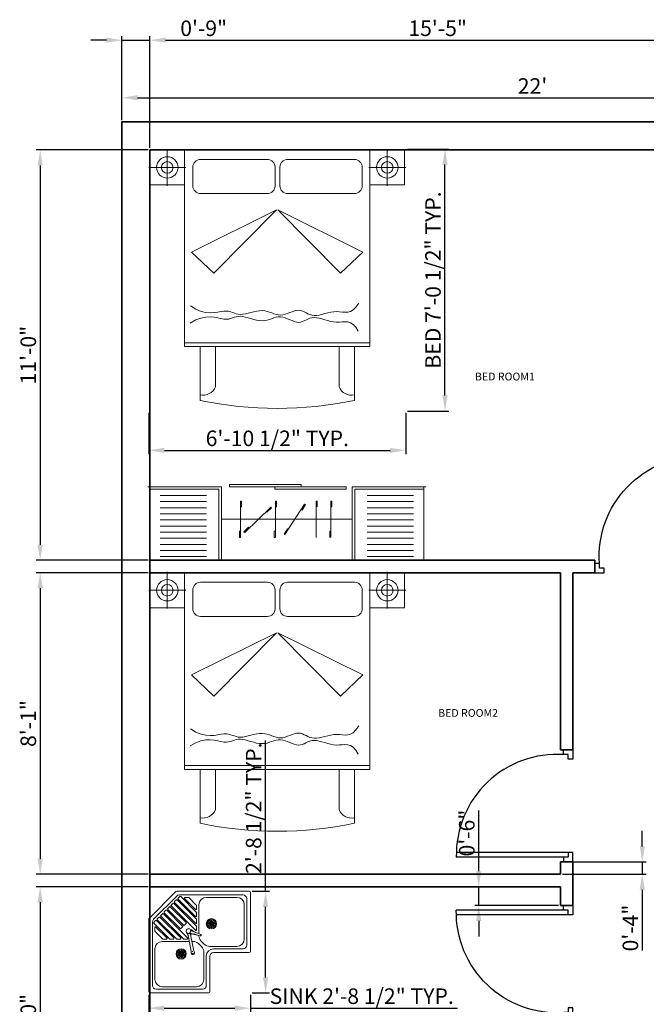
# Model space of a CAD drawing. Units: inches. Extents: x -24887 to 3061, y 1794 to 4919553.
# Tile 2 of 14: x 1576 to 1777, y 2047 to 2364. Entities that reach past the tile are written whole.
import ezdxf

# ---------------------------------------------------------------- set-up
doc = ezdxf.new("R2010")
doc.units = ezdxf.units.IN
for name, color, linetype, lineweight in [('A-ANNO-DIMS', 2, 'Continuous', 18), ('A-AREA-IDEN', 7, 'Continuous', 18), ('A-FLOR-FIXT', 9, 'Continuous', 18), ('A-FURN', 8, 'Continuous', 18), ('door', 4, 'Continuous', 25), ('wall', 7, 'Continuous', 35)]:
    doc.layers.add(name, color=color, linetype=linetype, lineweight=lineweight)
doc.styles.get("Standard").update_dxf_attribs({"font": 'arial.ttf'})
doc.dimstyles.new('ISO-25', dxfattribs={"dimtxt": 5, "dimasz": 5, "dimexe": 1.25, "dimexo": 0.625, "dimtad": 1, "dimdec": 1, "dimlunit": 3, "dimtxsty": 'Standard', "dimcen": 2.5, "dimadec": 0, "dimazin": 0, "dimtfac": 1, "dimtdec": 1, "dimtmove": 0, "dimatfit": 3, "dimfxl": 1, "dimarcsym": 0})

# ---------------------------------------------------------------- blocks, each defined once
blk = doc.blocks.new('A$C4F543DC7')
for p, q in [((0.013, 3.35, -0.169), (3.313, 3.35, -0.169)), ((0.463, 3.35, -0.169), (0.013, 3.35, -0.169)), ((0.013, 2.896, -0.169), (0.013, 3.35, -0.169)), ((0.013, 3.35, -0.169), (0.013, 2.896, -0.169)), ((0.238, 3.123, -0.439), (0.238, 3.361, -0.439)), ((0.463, 3.35, -0.169), (0.463, 0.8, -0.169)), ((2.863, 3.35, -0.169), (0.463, 3.35, -0.169)), ((0.463, 2.896, -0.169), (0.463, 3.35, -0.169)), ((2.863, 0.8, -0.169), (2.863, 3.35, -0.169)), ((2.863, 3.35, -0.169), (3.313, 3.35, -0.169)), ((2.863, 2.896, -0.169), (2.863, 3.35, -0.169)), ((3.089, 3.123, -0.439), (3.089, 3.361, -0.439)), ((3.313, 3.35, -0.169), (3.313, 2.896, -0.169)), ((3.313, 3.35, -0.169), (3.313, 2.896, -0.169)), ((1.535, 3.226, -0.169), (0.668, 3.226, -0.169)), ((2.664, 3.226, -0.169), (1.797, 3.226, -0.169)), ((0.238, 3.123, -0.439), (0, 3.123, -0.439)), ((0.238, 3.123, -0.439), (0.476, 3.123, -0.439)), ((0.238, 3.123, -0.439), (0.238, 2.885, -0.439)), ((0.568, 3.126, -0.169), (0.568, 2.884, -0.169)), ((1.635, 2.884, -0.169), (1.635, 3.126, -0.169)), ((1.697, 3.126, -0.169), (1.697, 2.884, -0.169)), ((2.764, 2.884, -0.169), (2.764, 3.126, -0.169)), ((3.089, 3.123, -0.439), (2.851, 3.123, -0.439)), ((3.089, 3.123, -0.439), (3.089, 2.885, -0.439)), ((3.089, 3.123, -0.439), (3.327, 3.123, -0.439)), ((0.463, 2.896, -0.169), (0.013, 2.896, -0.169)), ((0.013, 2.896, -0.169), (0.463, 2.896, -0.169)), ((0.463, 0.8, -0.169), (0.463, 2.896, -0.169)), ((2.863, 2.896, -0.169), (2.863, 0.8, -0.169)), ((3.313, 2.896, -0.169), (2.863, 2.896, -0.169)), ((3.313, 2.896, -0.169), (2.863, 2.896, -0.169)), ((0.668, 2.784, -0.169), (1.535, 2.784, -0.169)), ((1.797, 2.784, -0.169), (2.664, 2.784, -0.169)), ((1.653, 2.573, -0.169), (0.55, 2.025, -0.169)), ((0.841, 1.752, -0.169), (1.653, 2.573, -0.169)), ((2.481, 1.752, -0.169), (1.669, 2.573, -0.169)), ((1.669, 2.573, -0.169), (2.772, 2.025, -0.169)), ((0.55, 2.025, -0.169), (0.841, 1.752, -0.169)), ((2.772, 2.025, -0.169), (2.481, 1.752, -0.169)), ((0.537, 1.327, -0.169), (0.609, 1.284, -0.169)), ((0.609, 1.284, -0.169), (0.676, 1.257, -0.169)), ((2.613, 1.257, -0.169), (2.648, 1.277, -0.169)), ((2.648, 1.277, -0.169), (2.683, 1.312, -0.169)), ((2.683, 1.312, -0.169), (2.718, 1.364, -0.169)), ((0.607, 1.146, -0.169), (0.674, 1.171, -0.169)), ((0.674, 1.171, -0.169), (0.736, 1.183, -0.169)), ((0.676, 1.257, -0.169), (0.737, 1.243, -0.169)), ((0.736, 1.183, -0.169), (0.793, 1.185, -0.169)), ((0.737, 1.243, -0.169), (0.794, 1.239, -0.169)), ((0.793, 1.185, -0.169), (0.845, 1.18, -0.169)), ((0.794, 1.239, -0.169), (0.846, 1.242, -0.169)), ((0.845, 1.18, -0.169), (0.891, 1.172, -0.169)), ((0.846, 1.242, -0.169), (0.893, 1.249, -0.169)), ((0.891, 1.172, -0.169), (0.933, 1.163, -0.169)), ((0.893, 1.249, -0.169), (0.935, 1.256, -0.169)), ((0.933, 1.163, -0.169), (0.97, 1.156, -0.169)), ((0.935, 1.256, -0.169), (0.972, 1.261, -0.169)), ((0.97, 1.156, -0.169), (1.003, 1.155, -0.169)), ((0.972, 1.261, -0.169), (1.004, 1.262, -0.169)), ((1.003, 1.155, -0.169), (1.032, 1.158, -0.169)), ((1.004, 1.262, -0.169), (1.033, 1.258, -0.169)), ((1.032, 1.158, -0.169), (1.058, 1.164, -0.169)), ((1.033, 1.258, -0.169), (1.06, 1.251, -0.169)), ((1.058, 1.164, -0.169), (1.083, 1.172, -0.169)), ((1.06, 1.251, -0.169), (1.084, 1.242, -0.169)), ((1.083, 1.172, -0.169), (1.107, 1.18, -0.169)), ((1.084, 1.242, -0.169), (1.108, 1.234, -0.169)), ((1.107, 1.18, -0.169), (1.132, 1.187, -0.169)), ((1.108, 1.234, -0.169), (1.132, 1.226, -0.169)), ((1.132, 1.226, -0.169), (1.158, 1.22, -0.169)), ((1.132, 1.187, -0.169), (1.157, 1.192, -0.169)), ((1.157, 1.192, -0.169), (1.185, 1.193, -0.169)), ((1.158, 1.22, -0.169), (1.185, 1.218, -0.169)), ((1.185, 1.218, -0.169), (1.216, 1.22, -0.169)), ((1.185, 1.193, -0.169), (1.216, 1.19, -0.169)), ((1.216, 1.22, -0.169), (1.25, 1.226, -0.169)), ((1.216, 1.19, -0.169), (1.249, 1.183, -0.169)), ((1.249, 1.183, -0.169), (1.284, 1.173, -0.169)), ((1.25, 1.226, -0.169), (1.285, 1.235, -0.169)), ((1.284, 1.173, -0.169), (1.321, 1.163, -0.169)), ((1.285, 1.235, -0.169), (1.322, 1.244, -0.169)), ((1.321, 1.163, -0.169), (1.358, 1.152, -0.169)), ((1.322, 1.244, -0.169), (1.359, 1.253, -0.169)), ((1.358, 1.152, -0.169), (1.394, 1.143, -0.169)), ((1.359, 1.253, -0.169), (1.396, 1.261, -0.169)), ((1.396, 1.261, -0.169), (1.433, 1.266, -0.169)), ((1.433, 1.266, -0.169), (1.468, 1.268, -0.169)), ((1.468, 1.268, -0.169), (1.501, 1.264, -0.169)), ((1.501, 1.264, -0.169), (1.532, 1.257, -0.169)), ((1.531, 1.143, -0.169), (1.561, 1.152, -0.169)), ((1.532, 1.257, -0.169), (1.562, 1.247, -0.169)), ((1.561, 1.152, -0.169), (1.59, 1.162, -0.169)), ((1.562, 1.247, -0.169), (1.591, 1.237, -0.169)), ((1.59, 1.162, -0.169), (1.619, 1.172, -0.169)), ((1.591, 1.237, -0.169), (1.62, 1.226, -0.169)), ((1.619, 1.172, -0.169), (1.648, 1.18, -0.169)), ((1.62, 1.226, -0.169), (1.648, 1.217, -0.169)), ((1.648, 1.217, -0.169), (1.676, 1.211, -0.169)), ((1.648, 1.18, -0.169), (1.676, 1.185, -0.169)), ((1.676, 1.211, -0.169), (1.705, 1.209, -0.169)), ((1.676, 1.185, -0.169), (1.705, 1.186, -0.169)), ((1.705, 1.209, -0.169), (1.735, 1.212, -0.169)), ((1.705, 1.186, -0.169), (1.734, 1.182, -0.169)), ((1.734, 1.182, -0.169), (1.764, 1.173, -0.169)), ((1.735, 1.212, -0.169), (1.765, 1.22, -0.169)), ((1.764, 1.173, -0.169), (1.794, 1.162, -0.169)), ((1.765, 1.22, -0.169), (1.795, 1.23, -0.169)), ((1.794, 1.162, -0.169), (1.824, 1.149, -0.169)), ((1.795, 1.23, -0.169), (1.826, 1.242, -0.169)), ((1.824, 1.149, -0.169), (1.854, 1.137, -0.169)), ((1.826, 1.242, -0.169), (1.856, 1.253, -0.169)), ((1.856, 1.253, -0.169), (1.885, 1.263, -0.169)), ((1.885, 1.263, -0.169), (1.913, 1.27, -0.169)), ((1.913, 1.27, -0.169), (1.94, 1.272, -0.169)), ((1.94, 1.272, -0.169), (1.965, 1.269, -0.169)), ((1.965, 1.269, -0.169), (1.989, 1.262, -0.169)), ((1.989, 1.262, -0.169), (2.012, 1.251, -0.169)), ((2.012, 1.251, -0.169), (2.036, 1.239, -0.169)), ((2.034, 1.145, -0.169), (2.059, 1.157, -0.169)), ((2.036, 1.239, -0.169), (2.06, 1.227, -0.169)), ((2.059, 1.157, -0.169), (2.084, 1.167, -0.169)), ((2.06, 1.227, -0.169), (2.085, 1.216, -0.169)), ((2.084, 1.167, -0.169), (2.111, 1.174, -0.169)), ((2.085, 1.216, -0.169), (2.112, 1.208, -0.169)), ((2.111, 1.174, -0.169), (2.14, 1.177, -0.169)), ((2.112, 1.208, -0.169), (2.141, 1.204, -0.169)), ((2.14, 1.177, -0.169), (2.172, 1.175, -0.169)), ((2.141, 1.204, -0.169), (2.172, 1.205, -0.169)), ((2.172, 1.205, -0.169), (2.206, 1.21, -0.169)), ((2.172, 1.175, -0.169), (2.206, 1.169, -0.169)), ((2.206, 1.21, -0.169), (2.242, 1.218, -0.169)), ((2.206, 1.169, -0.169), (2.241, 1.16, -0.169)), ((2.241, 1.16, -0.169), (2.278, 1.149, -0.169)), ((2.242, 1.218, -0.169), (2.279, 1.228, -0.169)), ((2.278, 1.149, -0.169), (2.316, 1.138, -0.169)), ((2.279, 1.228, -0.169), (2.317, 1.238, -0.169)), ((2.317, 1.238, -0.169), (2.356, 1.246, -0.169)), ((2.356, 1.246, -0.169), (2.394, 1.253, -0.169)), ((2.394, 1.253, -0.169), (2.433, 1.255, -0.169)), ((2.433, 1.255, -0.169), (2.47, 1.253, -0.169)), ((2.47, 1.253, -0.169), (2.506, 1.249, -0.169)), ((2.506, 1.249, -0.169), (2.542, 1.246, -0.169)), ((2.542, 1.246, -0.169), (2.578, 1.248, -0.169)), ((2.578, 1.248, -0.169), (2.613, 1.257, -0.169)), ((0.533, 1.105, -0.169), (0.607, 1.146, -0.169)), ((1.394, 1.143, -0.169), (1.431, 1.137, -0.169)), ((1.431, 1.137, -0.169), (1.466, 1.135, -0.169)), ((1.466, 1.135, -0.169), (1.499, 1.137, -0.169)), ((1.499, 1.137, -0.169), (1.531, 1.143, -0.169)), ((1.854, 1.137, -0.169), (1.883, 1.126, -0.169)), ((1.883, 1.126, -0.169), (1.911, 1.119, -0.169)), ((1.911, 1.119, -0.169), (1.937, 1.115, -0.169)), ((1.937, 1.115, -0.169), (1.963, 1.118, -0.169)), ((1.963, 1.118, -0.169), (1.987, 1.124, -0.169)), ((1.987, 1.124, -0.169), (2.011, 1.134, -0.169)), ((2.011, 1.134, -0.169), (2.034, 1.145, -0.169)), ((2.316, 1.138, -0.169), (2.354, 1.128, -0.169)), ((2.354, 1.128, -0.169), (2.392, 1.121, -0.169)), ((2.392, 1.121, -0.169), (2.43, 1.117, -0.169)), ((2.43, 1.117, -0.169), (2.468, 1.118, -0.169)), ((2.468, 1.118, -0.169), (2.504, 1.121, -0.169)), ((2.504, 1.121, -0.169), (2.54, 1.123, -0.169)), ((2.54, 1.123, -0.169), (2.576, 1.12, -0.169)), ((2.576, 1.12, -0.169), (2.611, 1.109, -0.169)), ((2.611, 1.109, -0.169), (2.645, 1.088, -0.169)), ((2.645, 1.088, -0.169), (2.679, 1.052, -0.169)), ((2.679, 1.052, -0.169), (2.712, 0.999, -0.169)), ((0.463, 0.85, -0.169), (2.863, 0.85, -0.169)), ((0.463, 0.8, -0.169), (2.863, 0.8, -0.169)), ((0.663, 0.8, -0.169), (0.463, 0.8, -0.169)), ((0.663, 0.8, -0.169), (2.663, 0.8, -0.169)), ((0.663, 0.104, -0.169), (0.663, 0.8, -0.169)), ((0.663, 0.104, -0.169), (0.663, 0.8, -0.169)), ((0.863, 0.281, -0.169), (0.863, 0.8, -0.169)), ((2.463, 0.8, -0.169), (2.463, 0.281, -0.169)), ((2.863, 0.8, -0.169), (2.663, 0.8, -0.169)), ((2.663, 0.8, -0.169), (2.663, 0.104, -0.169)), ((2.663, 0.8, -0.169), (2.663, 0.104, -0.169))]:
    blk.add_line(p, q)
for centre, radius in [((0.238, 3.123, -0.439), 0.139), ((0.238, 3.123, -0.439), 0.075), ((3.089, 3.123, -0.439), 0.139), ((3.089, 3.123, -0.439), 0.075)]:
    blk.add_circle(centre, radius)
for centre, radius, start, end in [((0.668, 3.126, -0.169), 0.1, 90, 180), ((1.535, 3.126, -0.169), 0.1, 0, 90), ((1.797, 3.126, -0.169), 0.1, 90, 180), ((2.664, 3.126, -0.169), 0.1, 0, 90), ((0.668, 2.884, -0.169), 0.1, 180, 270), ((1.535, 2.884, -0.169), 0.1, 270, 0), ((1.797, 2.884, -0.169), 0.1, 180, 270), ((2.664, 2.884, -0.169), 0.1, 270, 0), ((0.699, 0.347, -0.169), 0.177, 258.2616, 338.032), ((2.627, 0.347, -0.169), 0.177, 201.968, 281.7384), ((1.663, 4.86, -0.169), 4.86, 258.1252, 281.8748), ((1.663, 4.86, -0.169), 4.86, 258.1252, 281.8748)]:
    blk.add_arc(centre, radius, start, end)
blk = doc.blocks.new('A$C34930FF8')
at = {"ltscale": 0.05}
for p, q in [((0, 2252.4), (0, 16.8)), ((600, 2252.4), (0, 2252.4)), ((185.4, 1513), (185.4, 1521.5)), ((227.1, 1479.2), (233.2, 1485.2)), ((237.7, 1513), (237.7, 1521.5)), ((436.7, 1513), (436.7, 1504.4)), ((482.5, 1513), (482.5, 1504.4)), ((263.6, 1441.7), (269.7, 1447.7)), ((398.2, 1303.6), (392.1, 1297.6)), ((185.4, 1229.1), (185.4, 1237.7)), ((237.7, 1229.1), (237.7, 1237.7)), ((434.8, 1266.1), (428.7, 1260.1)), ((436.7, 1228.2), (436.7, 1219.7)), ((482.5, 1228.2), (482.5, 1219.7)), ((209.5, 1150.1), (214.1, 1157.3)), ((253.5, 1121.8), (258.1, 1129)), ((415.3, 1017.6), (410.6, 1010.5)), ((459.3, 989.3), (454.7, 982.1)), ((482.5, 894.9), (482.5, 886.3)), ((237.7, 775.3), (237.7, 783.9)), ((436.7, 775.3), (436.7, 766.8)), ((482.5, 775.3), (482.5, 766.8)), ((600, 16.8), (0, 16.8))]:
    blk.add_line(p, q, dxfattribs=at)
for p, q in [((580, 1690.9), (580, 2252.4)), ((600, 1669.3), (600, 2269.3)), ((30, 1790.9), (30, 2169.3)), ((80, 1790.9), (80, 2169.3)), ((130, 1790.9), (130, 2169.3)), ((180, 1790.9), (180, 2169.3)), ((230, 1790.9), (230, 2169.3)), ((280, 1790.9), (280, 2169.3)), ((330, 1790.9), (330, 2169.3)), ((380, 1790.9), (380, 2169.3)), ((430, 1790.9), (430, 2169.3)), ((480, 1790.9), (480, 2169.3)), ((530, 1790.9), (530, 2169.3)), ((580, 1690.9), (0, 1690.9)), ((600, 1669.3), (0, 1669.3)), ((335.4, 1666.1), (335.4, 603.1)), ((600, 1603.3), (620, 1603.3)), ((600, 1018.7), (600, 1603.3)), ((620, 1603.3), (620, 1018.7)), ((237.7, 1521.5), (185.4, 1521.5)), ((482.5, 1513), (185.4, 1513)), ((434.8, 1266.1), (227.4, 1478.9)), ((269.7, 1447.7), (233.2, 1485.2)), ((436.7, 1504.4), (482.5, 1504.4)), ((428.7, 1260.1), (392.1, 1297.6)), ((237.7, 1237.7), (185.4, 1237.7)), ((482.5, 1228.2), (185.4, 1228.2)), ((436.7, 1219.7), (482.5, 1219.7)), ((600, 1233.4), (580, 1233.4)), ((580, 1233.4), (580, 648.7)), ((600, 648.7), (600, 1233.4)), ((459.3, 989.3), (209.5, 1150.1)), ((258.1, 1129), (214.1, 1157.3)), ((454.7, 982.1), (410.6, 1010.5)), ((620, 1018.7), (600, 1018.7)), ((482.5, 894.9), (185.4, 894.9)), ((436.7, 886.3), (482.5, 886.3)), ((237.7, 783.9), (185.4, 783.9)), ((482.5, 775.3), (185.4, 775.3)), ((436.7, 766.8), (482.5, 766.8)), ((580, 648.7), (600, 648.7)), ((600, 600), (0, 600)), ((580, 578.3), (0, 578.3)), ((580, 578.3), (580, 16.8)), ((600, 600), (600, 0)), ((30, 478.3), (30, 100)), ((80, 478.3), (80, 100)), ((130, 478.3), (130, 100)), ((180, 478.3), (180, 100)), ((230, 478.3), (230, 100)), ((280, 478.3), (280, 100)), ((330, 478.3), (330, 100)), ((380, 478.3), (380, 100)), ((430, 478.3), (430, 100)), ((480, 478.3), (480, 100)), ((530, 478.3), (530, 100))]:
    blk.add_line(p, q)
blk = doc.blocks.new('A$C4E531579')
for p, q in [((222.1, 827.1), (2.9, 607.9)), ((229.1, 830), (820, 830)), ((830, 820), (830, 340)), ((228.6, 791.2), (38.8, 601.4)), ((197.4, 731.6), (183.2, 717.5)), ((388.5, 547.5), (204.4, 731.6)), ((225.6, 759.9), (211.5, 745.8)), ((381.5, 568.7), (211.5, 738.7)), ((388.5, 604.1), (232.7, 759.9)), ((253.9, 788.2), (239.8, 774.1)), ((381.5, 625.3), (239.8, 767)), ((249.9, 800), (770, 800)), ((388.5, 660.7), (261, 788.2)), ((381.5, 681.9), (291.9, 771.5)), ((295.4, 780), (323.7, 780)), ((388.5, 717.2), (327.2, 778.5)), ((720, 780), (470, 780)), ((800, 770), (800, 390)), ((98.4, 632.6), (112.5, 646.8)), ((317.8, 448.5), (119.6, 646.8)), ((126.6, 660.9), (140.8, 675.1)), ((255.6, 524.9), (126.6, 653.9)), ((276.8, 546.1), (147.9, 675.1)), ((169.1, 703.4), (154.9, 689.2)), ((283.9, 553.2), (154.9, 682.1)), ((305.1, 574.4), (176.1, 703.4)), ((381.5, 512.2), (183.2, 710.4)), ((390, 713.7), (390, 685.4)), ((390, 657.1), (390, 628.8)), ((410, 720), (410, 483.9)), ((780, 440), (780, 720)), ((0, 10), (0, 600.9)), ((30, 60), (30, 580.1)), ((41.8, 576.1), (55.9, 590.2)), ((169.3, 441.5), (41.8, 569)), ((204.7, 448.5), (63, 590.2)), ((70.1, 604.4), (84.2, 618.5)), ((225.9, 441.5), (70.1, 597.3)), ((261.3, 448.5), (91.3, 618.5)), ((282.5, 441.5), (98.4, 625.6)), ((305.1, 567.3), (291, 553.2)), ((390, 600.6), (390, 572.3)), ((50, 534.6), (50, 506.3)), ((112.8, 441.5), (51.5, 502.8)), ((148.1, 448.5), (58.5, 538.1)), ((262.7, 524.9), (276.8, 539)), ((390, 544), (390, 515.7)), ((110, 420), (331.5, 420)), ((116.3, 440), (144.6, 440)), ((172.9, 440), (201.2, 440)), ((229.4, 440), (257.7, 440)), ((286, 440), (314.3, 440)), ((344.7, 353.4), (324.5, 455.5)), ((344.5, 460.1), (364.9, 357.1)), ((352.4, 420), (363.9, 420)), ((406.4, 402.4), (432.4, 376.4)), ((410, 468.8), (410, 466.1)), ((427.6, 423.6), (453.6, 397.6)), ((50, 110), (50, 360)), ((450, 333.9), (450, 110)), ((496.1, 380), (720, 380)), ((530, 360), (770, 360)), ((530, 330), (820, 330)), ((470, 300), (470, 60)), ((500, 300), (500, 10)), ((440, 30), (60, 30)), ((390, 50), (110, 50)), ((490, 0), (10, 0))]:
    blk.add_line(p, q)
for centre, radius in [((511.9, 565), 41.9), ((511.9, 565), 34.4), ((511.9, 565), 5.37), ((265, 318.1), 41.9), ((265, 318.1), 34.4), ((265, 318.1), 5.37)]:
    blk.add_circle(centre, radius)
for centre, radius, start, end in [((229.1, 820), 10, 90, 135), ((820, 820), 10, 0, 90), ((200.9, 728.1), 5, 45, 135), ((215, 742.2), 5, 135, 225), ((229.2, 756.4), 5, 45, 135), ((249.9, 770), 30, 90, 135), ((243.3, 770.5), 5, 135, 225), ((257.5, 784.7), 5, 45, 135), ((295.4, 775), 5, 90, 225), ((323.7, 775), 5, 45, 90), ((470, 720), 60, 90, 180), ((720, 720), 60, 0, 90), ((770, 770), 30, 0, 90), ((116, 643.3), 5, 45, 135), ((130.2, 657.4), 5, 135, 225), ((144.3, 671.5), 5, 45, 135), ((158.5, 685.7), 5, 135, 225), ((172.6, 699.8), 5, 45, 135), ((186.7, 714), 5, 135, 225), ((385, 685.4), 5, 225, 0), ((385, 713.7), 5, 0, 45), ((385, 657.1), 5, 0, 45), ((10, 600.9), 10, 135, 180), ((60, 580.1), 30, 135, 180), ((45.3, 572.5), 5, 135, 225), ((59.5, 586.7), 5, 45, 135), ((73.6, 600.8), 5, 135, 225), ((87.8, 615), 5, 45, 135), ((101.9, 629.1), 5, 135, 225), ((301.6, 570.8), 5, 315, 45), ((385, 628.8), 5, 225, 0), ((385, 572.3), 5, 225, 0), ((385, 600.6), 5, 0, 45), ((55, 534.6), 5, 45, 180), ((55, 506.3), 5, 180, 225), ((259.2, 528.4), 5, 225, 315), ((273.3, 542.6), 5, 315, 45), ((287.4, 556.7), 5, 225, 315), ((325.6, 504.4), 20, 52.72293, 268.78568), ((226.1, 437.3), 100, 10.4867, 33.97381), ((282.9, 16.5), 469.7, 72.94476, 84.83287), ((326.2, 504.9), 16.2, 278.92915, 32.15573), ((305.7, 211.8), 277.4, 72.23491, 84.23498), ((583, 916.9), 466.4, 238.27092, 250.20216), ((368.8, 476.8), 29.3, 168.25085, 191.99309), ((479.5, 750.1), 274.6, 239.9645, 252.02573), ((385, 515.7), 5, 225, 0), ((385, 544), 5, 0, 45), ((110, 360), 60, 90, 180), ((116.3, 445), 5, 225, 270), ((144.6, 445), 5, 270, 45), ((172.9, 445), 5, 225, 270), ((201.2, 445), 5, 270, 45), ((229.4, 445), 5, 225, 270), ((257.7, 445), 5, 270, 45), ((286, 445), 5, 225, 270), ((314.3, 445), 5, 270, 45), ((296.1, 462.7), 29.3, 9.84672, 38.35374), ((442.8, 478.3), 100, 177.65932, 190.48676), ((363.9, 360), 60, 45, 90), ((470, 466.1), 60, 180, 225), ((422.7, 471.9), 6.64, 252.6444, 68.86421), ((420.8, 471.6), 4.91, 314.25167, 37.23492), ((720, 440), 60, 270, 0), ((246.4, 335.2), 100, 355.98426, 10.4867), ((360, 327.2), 13.9, 175.98426, 24.98921), ((359.8, 327.5), 8.12, 180.36355, 342.44433), ((359, 332), 7.59, 72.42297, 131.67578), ((463.2, 375.3), 100, 190.48676, 204.98921), ((390, 333.9), 60, 0, 45), ((496.1, 440), 60, 225, 270), ((530, 300), 60, 90, 180), ((530, 300), 30, 90, 180), ((770, 390), 30, 270, 0), ((820, 340), 10, 270, 0), ((110, 110), 60, 180, 270), ((390, 110), 60, 270, 0), ((10, 10), 10, 180, 270), ((60, 60), 30, 180, 270), ((440, 60), 30, 270, 0), ((490, 10), 10, 270, 0)]:
    blk.add_arc(centre, radius, start, end)
at = {"extrusion": (0, -1e-16, -1)}
for centre, major_axis in [((492, 565), (14.5, 0)), ((511.9, 545.1), (0, 14.5))]:
    blk.add_ellipse(centre, major_axis=major_axis, ratio=0.137964, dxfattribs=at)
at = {"extrusion": (-1e-16, -2e-16, -1)}
blk.add_ellipse((494.7, 574.9), major_axis=(12.6, -7.2), ratio=0.137964, dxfattribs=at)
at = {"extrusion": (0, -2e-16, -1)}
for centre, major_axis in [((494.7, 555.1), (12.6, 7.2)), ((529.1, 574.9), (-12.6, -7.2))]:
    blk.add_ellipse(centre, major_axis=major_axis, ratio=0.137964, dxfattribs=at)
at = {"extrusion": (0, 0, -1)}
for centre, major_axis in [((501.9, 582.2), (7.2, -12.6)), ((511.9, 584.9), (0, -14.5)), ((521.8, 547.8), (-7.2, 12.6))]:
    blk.add_ellipse(centre, major_axis=major_axis, ratio=0.137964, dxfattribs=at)
at = {"extrusion": (3e-16, -1e-16, -1)}
blk.add_ellipse((521.8, 582.2), major_axis=(-7.2, -12.6), ratio=0.137964, dxfattribs=at)
at = {"extrusion": (-1e-16, -1e-16, -1)}
blk.add_ellipse((529.1, 555.1), major_axis=(-12.6, 7.2), ratio=0.137964, dxfattribs=at)
at = {"extrusion": (1e-16, -1e-16, -1)}
blk.add_ellipse((531.7, 565), major_axis=(-14.5, 0), ratio=0.137964, dxfattribs=at)
at = {"extrusion": (-3e-16, 1e-16, -1)}
blk.add_ellipse((501.9, 547.8), major_axis=(7.2, 12.6), ratio=0.137964, dxfattribs=at)
for centre, major_axis in [((247.8, 328.1), (12.6, -7.2)), ((255.1, 335.3), (7.2, -12.6)), ((265, 338), (0, -14.5)), ((274.9, 335.3), (-7.2, -12.6)), ((282.2, 328.1), (-12.6, -7.2)), ((245.1, 318.1), (14.5, 0)), ((247.8, 308.2), (12.6, 7.2)), ((255.1, 300.9), (7.2, 12.6)), ((265, 298.3), (0, 14.5)), ((274.9, 300.9), (-7.2, 12.6)), ((282.2, 308.2), (-12.6, 7.2)), ((284.9, 318.1), (-14.5, 0))]:
    blk.add_ellipse(centre, major_axis=major_axis, ratio=0.137964)
blk = doc.blocks.new('*D28')
at = {"layer": 'A-ANNO-DIMS', "color": 0, "lineweight": -2, "transparency": 16777216}
for p, q in [((1608.43, 2331.48), (1608.43, 2339.9)), ((1613.43, 2338.65), (1867.43, 2338.65)), ((1872.43, 2331.48), (1872.43, 2339.9))]:
    blk.add_line(p, q, dxfattribs=at)
at = {"layer": 'A-ANNO-DIMS', "color": 0, "transparency": 16777216}
for points in [[(1613.43, 2339.48), (1613.43, 2337.81), (1608.43, 2338.65)], [(1867.43, 2339.48), (1867.43, 2337.81), (1872.43, 2338.65)]]:
    blk.add_solid(points, dxfattribs=at)
at = {"layer": 'Defpoints', "color": 0, "transparency": 16777216}
for p in [(1872.43, 2338.65), (1608.43, 2330.86), (1872.43, 2330.86)]:
    blk.add_point(p, dxfattribs=at)
at = {"layer": 'A-ANNO-DIMS', "color": 0, "transparency": 16777216, "insert": (1740.43, 2341.78), "char_height": 5, "attachment_point": 5}
blk.add_mtext("22'", dxfattribs=at)
blk = doc.blocks.new('DOOR-SINGLE-36IN')
for p, q in [((34.5, 36), (37.5, 36)), ((34.5, 34.5), (34.5, 36)), ((37.5, 36), (37.5, 33)), ((36, 34.5), (34.5, 34.5)), ((36, 33), (36, 34.5)), ((37.5, 33), (36, 33)), ((36, 3), (0, 3)), ((36, 1.5), (0, 1.5)), ((36, 1.5), (34.5, 1.5)), ((34.5, 1.5), (34.5, 0)), ((34.5, 0), (37.5, 0)), ((37.5, 3), (36, 3)), ((36, 3), (36, 1.5)), ((37.5, 0), (37.5, 3))]:
    blk.add_line(p, q)
blk.add_arc((32.32, 2.25), 32.32, 86.1244, 181.3295)
blk = doc.blocks.new('*D40')
at = {"layer": 'A-ANNO-DIMS', "color": 0, "lineweight": -2, "transparency": 16777216}
for p, q in [((1700.28, 2322.14), (1713.54, 2322.14)), ((1712.29, 2242.87), (1712.29, 2317.14)), ((1700.28, 2237.87), (1713.54, 2237.87))]:
    blk.add_line(p, q, dxfattribs=at)
at = {"layer": 'A-ANNO-DIMS', "color": 0, "transparency": 16777216}
for points in [[(1711.46, 2317.14), (1713.13, 2317.14), (1712.29, 2322.14)], [(1711.46, 2242.87), (1713.13, 2242.87), (1712.29, 2237.87)]]:
    blk.add_solid(points, dxfattribs=at)
at = {"layer": 'Defpoints', "color": 0, "transparency": 16777216}
for p in [(1699.65, 2322.14), (1712.29, 2322.14), (1699.65, 2237.87)]:
    blk.add_point(p, dxfattribs=at)
at = {"layer": 'A-ANNO-DIMS', "color": 0, "transparency": 16777216, "insert": (1709.08, 2280.01), "char_height": 5, "attachment_point": 5, "rotation": 90}
blk.add_mtext('BED 7\'-0 1/2" TYP.', dxfattribs=at)
blk = doc.blocks.new('*D41')
at = {"layer": 'A-ANNO-DIMS', "color": 0, "lineweight": -2, "transparency": 16777216}
for p, q in [((1617.1, 2237.24), (1617.1, 2223.98)), ((1699.65, 2237.24), (1699.65, 2223.98)), ((1622.1, 2225.23), (1694.65, 2225.23))]:
    blk.add_line(p, q, dxfattribs=at)
at = {"layer": 'A-ANNO-DIMS', "color": 0, "transparency": 16777216}
for points in [[(1622.1, 2226.06), (1622.1, 2224.4), (1617.1, 2225.23)], [(1694.65, 2226.06), (1694.65, 2224.4), (1699.65, 2225.23)]]:
    blk.add_solid(points, dxfattribs=at)
at = {"layer": 'Defpoints', "color": 0, "transparency": 16777216}
for p in [(1617.1, 2237.87), (1699.65, 2237.87), (1699.65, 2225.23)]:
    blk.add_point(p, dxfattribs=at)
at = {"layer": 'A-ANNO-DIMS', "color": 0, "transparency": 16777216, "insert": (1658.38, 2228.44), "char_height": 5, "attachment_point": 5}
blk.add_mtext('6\'-10 1/2" TYP.', dxfattribs=at)
blk = doc.blocks.new('*D54')
at = {"layer": 'A-ANNO-DIMS', "color": 0, "lineweight": -2, "transparency": 16777216}
for p, q in [((1617.04, 2050.09), (1617.04, 2044.56)), ((1649.71, 2050.09), (1649.71, 2044.56)), ((1622.04, 2045.81), (1644.71, 2045.81)), ((1649.71, 2045.81), (1716.31, 2045.81))]:
    blk.add_line(p, q, dxfattribs=at)
at = {"layer": 'A-ANNO-DIMS', "color": 0, "transparency": 16777216}
for points in [[(1622.04, 2046.65), (1622.04, 2044.98), (1617.04, 2045.81)], [(1644.71, 2046.65), (1644.71, 2044.98), (1649.71, 2045.81)]]:
    blk.add_solid(points, dxfattribs=at)
at = {"layer": 'Defpoints', "color": 0, "transparency": 16777216}
for p in [(1617.04, 2050.72), (1649.71, 2050.72), (1649.71, 2045.81)]:
    blk.add_point(p, dxfattribs=at)
at = {"layer": 'A-ANNO-DIMS', "color": 0, "transparency": 16777216, "insert": (1685.51, 2049.02), "char_height": 5, "attachment_point": 5}
blk.add_mtext('SINK 2\'-8 1/2" TYP.', dxfattribs=at)
blk = doc.blocks.new('*D55')
at = {"layer": 'A-ANNO-DIMS', "color": 0, "lineweight": -2, "transparency": 16777216}
for p, q in [((1654.62, 2083.39), (1654.62, 2131.86)), ((1650.34, 2083.39), (1655.87, 2083.39)), ((1654.62, 2055.72), (1654.62, 2078.39)), ((1650.34, 2050.72), (1655.87, 2050.72))]:
    blk.add_line(p, q, dxfattribs=at)
at = {"layer": 'A-ANNO-DIMS', "color": 0, "transparency": 16777216}
for points in [[(1653.78, 2078.39), (1655.45, 2078.39), (1654.62, 2083.39)], [(1653.78, 2055.72), (1655.45, 2055.72), (1654.62, 2050.72)]]:
    blk.add_solid(points, dxfattribs=at)
at = {"layer": 'Defpoints', "color": 0, "transparency": 16777216}
for p in [(1649.71, 2083.39), (1654.62, 2083.39), (1649.71, 2050.72)]:
    blk.add_point(p, dxfattribs=at)
at = {"layer": 'A-ANNO-DIMS', "color": 0, "transparency": 16777216, "insert": (1651.41, 2110.12), "char_height": 5, "attachment_point": 5, "rotation": 90}
blk.add_mtext('2\'-8 1/2" TYP.', dxfattribs=at)
blk = doc.blocks.new('*D66')
at = {"layer": 'A-ANNO-DIMS', "color": 0, "lineweight": -2, "transparency": 16777216}
for p, q in [((1603.43, 2357.16), (1598.43, 2357.16)), ((1608.43, 2331.48), (1608.43, 2358.41)), ((1608.43, 2357.16), (1617.43, 2357.16)), ((1617.43, 2322.48), (1617.43, 2358.41)), ((1622.43, 2357.16), (1641.97, 2357.16))]:
    blk.add_line(p, q, dxfattribs=at)
at = {"layer": 'A-ANNO-DIMS', "color": 0, "transparency": 16777216}
for points in [[(1603.43, 2357.99), (1603.43, 2356.33), (1608.43, 2357.16)], [(1622.43, 2357.99), (1622.43, 2356.33), (1617.43, 2357.16)]]:
    blk.add_solid(points, dxfattribs=at)
at = {"layer": 'Defpoints', "color": 0, "transparency": 16777216}
for p in [(1617.43, 2357.16), (1608.43, 2330.86), (1617.43, 2321.86)]:
    blk.add_point(p, dxfattribs=at)
at = {"layer": 'A-ANNO-DIMS', "color": 0, "transparency": 16777216, "insert": (1634.7, 2360.34), "char_height": 5, "attachment_point": 5}
blk.add_mtext('0\'-9"', dxfattribs=at)
blk = doc.blocks.new('*D67')
at = {"layer": 'A-ANNO-DIMS', "color": 0, "lineweight": -2, "transparency": 16777216}
for p, q in [((1617.43, 2322.48), (1617.43, 2358.41)), ((1622.43, 2357.16), (1797.43, 2357.16)), ((1802.43, 2322.48), (1802.43, 2358.41))]:
    blk.add_line(p, q, dxfattribs=at)
at = {"layer": 'A-ANNO-DIMS', "color": 0, "transparency": 16777216}
for points in [[(1622.43, 2357.99), (1622.43, 2356.33), (1617.43, 2357.16)], [(1797.43, 2357.99), (1797.43, 2356.33), (1802.43, 2357.16)]]:
    blk.add_solid(points, dxfattribs=at)
at = {"layer": 'Defpoints', "color": 0, "transparency": 16777216}
for p in [(1802.43, 2357.16), (1617.43, 2321.86), (1802.43, 2321.86)]:
    blk.add_point(p, dxfattribs=at)
at = {"layer": 'A-ANNO-DIMS', "color": 0, "transparency": 16777216, "insert": (1709.93, 2360.34), "char_height": 5, "attachment_point": 5}
blk.add_mtext('15\'-5"', dxfattribs=at)
blk = doc.blocks.new('*D71')
at = {"layer": 'A-ANNO-DIMS', "color": 0, "lineweight": -2, "transparency": 16777216}
for p, q in [((1616.81, 2321.86), (1580.88, 2321.86)), ((1582.13, 2316.86), (1582.13, 2194.86)), ((1616.81, 2189.86), (1580.88, 2189.86))]:
    blk.add_line(p, q, dxfattribs=at)
at = {"layer": 'A-ANNO-DIMS', "color": 0, "transparency": 16777216}
for points in [[(1581.3, 2316.86), (1582.96, 2316.86), (1582.13, 2321.86)], [(1581.3, 2194.86), (1582.96, 2194.86), (1582.13, 2189.86)]]:
    blk.add_solid(points, dxfattribs=at)
at = {"layer": 'Defpoints', "color": 0, "transparency": 16777216}
for p in [(1617.43, 2321.86), (1582.13, 2189.86), (1617.43, 2189.86)]:
    blk.add_point(p, dxfattribs=at)
at = {"layer": 'A-ANNO-DIMS', "color": 0, "transparency": 16777216, "insert": (1578.95, 2255.86), "char_height": 5, "attachment_point": 5, "rotation": 90}
blk.add_mtext('11\'-0"', dxfattribs=at)
blk = doc.blocks.new('*D72')
at = {"layer": 'A-ANNO-DIMS', "color": 0, "lineweight": -2, "transparency": 16777216}
for p, q in [((1616.81, 2185.86), (1580.88, 2185.86)), ((1582.13, 2180.86), (1582.13, 2093.86)), ((1616.81, 2088.86), (1580.88, 2088.86))]:
    blk.add_line(p, q, dxfattribs=at)
at = {"layer": 'A-ANNO-DIMS', "color": 0, "transparency": 16777216}
for points in [[(1581.3, 2180.86), (1582.96, 2180.86), (1582.13, 2185.86)], [(1581.3, 2093.86), (1582.96, 2093.86), (1582.13, 2088.86)]]:
    blk.add_solid(points, dxfattribs=at)
at = {"layer": 'Defpoints', "color": 0, "transparency": 16777216}
for p in [(1617.43, 2185.86), (1582.13, 2088.86), (1617.43, 2088.86)]:
    blk.add_point(p, dxfattribs=at)
at = {"layer": 'A-ANNO-DIMS', "color": 0, "transparency": 16777216, "insert": (1578.95, 2137.36), "char_height": 5, "attachment_point": 5, "rotation": 90}
blk.add_mtext('8\'-1"', dxfattribs=at)
blk = doc.blocks.new('*D73')
at = {"layer": 'A-ANNO-DIMS', "color": 0, "lineweight": -2, "transparency": 16777216}
for p, q in [((1616.81, 2084.86), (1580.88, 2084.86)), ((1582.13, 2079.86), (1582.13, 2005.86)), ((1616.81, 2000.86), (1580.88, 2000.86))]:
    blk.add_line(p, q, dxfattribs=at)
at = {"layer": 'A-ANNO-DIMS', "color": 0, "transparency": 16777216}
for points in [[(1581.3, 2079.86), (1582.96, 2079.86), (1582.13, 2084.86)], [(1581.3, 2005.86), (1582.96, 2005.86), (1582.13, 2000.86)]]:
    blk.add_solid(points, dxfattribs=at)
at = {"layer": 'Defpoints', "color": 0, "transparency": 16777216}
for p in [(1617.43, 2084.86), (1582.13, 2000.86), (1617.43, 2000.86)]:
    blk.add_point(p, dxfattribs=at)
at = {"layer": 'A-ANNO-DIMS', "color": 0, "transparency": 16777216, "insert": (1578.95, 2042.86), "char_height": 5, "attachment_point": 5, "rotation": 90}
blk.add_mtext('7\'-0"', dxfattribs=at)
blk = doc.blocks.new('*D81')
at = {"layer": 'A-ANNO-DIMS', "color": 0, "lineweight": -2, "transparency": 16777216}
for p, q in [((1775.73, 2097.86), (1775.73, 2102.86)), ((1750.06, 2092.86), (1776.98, 2092.86)), ((1775.73, 2092.86), (1775.73, 2088.86)), ((1750.06, 2088.86), (1776.98, 2088.86)), ((1775.73, 2083.86), (1775.73, 2064.32))]:
    blk.add_line(p, q, dxfattribs=at)
at = {"layer": 'A-ANNO-DIMS', "color": 0, "transparency": 16777216}
for points in [[(1774.9, 2097.86), (1776.56, 2097.86), (1775.73, 2092.86)], [(1774.9, 2083.86), (1776.56, 2083.86), (1775.73, 2088.86)]]:
    blk.add_solid(points, dxfattribs=at)
at = {"layer": 'Defpoints', "color": 0, "transparency": 16777216}
for p in [(1749.43, 2092.86), (1749.43, 2088.86), (1775.73, 2088.86)]:
    blk.add_point(p, dxfattribs=at)
at = {"layer": 'A-ANNO-DIMS', "color": 0, "transparency": 16777216, "insert": (1772.55, 2071.59), "char_height": 5, "attachment_point": 5, "rotation": 90}
blk.add_mtext('0\'-4"', dxfattribs=at)
blk = doc.blocks.new('*D82')
at = {"layer": 'A-ANNO-DIMS', "color": 0, "lineweight": -2, "transparency": 16777216}
for p, q in [((1723.13, 2089.86), (1723.13, 2109.4)), ((1748.81, 2084.86), (1721.88, 2084.86)), ((1723.13, 2078.86), (1723.13, 2084.86)), ((1748.81, 2078.86), (1721.88, 2078.86)), ((1723.13, 2073.86), (1723.13, 2068.86))]:
    blk.add_line(p, q, dxfattribs=at)
at = {"layer": 'A-ANNO-DIMS', "color": 0, "transparency": 16777216}
for points in [[(1722.3, 2089.86), (1723.96, 2089.86), (1723.13, 2084.86)], [(1722.3, 2073.86), (1723.96, 2073.86), (1723.13, 2078.86)]]:
    blk.add_solid(points, dxfattribs=at)
at = {"layer": 'Defpoints', "color": 0, "transparency": 16777216}
for p in [(1723.13, 2084.86), (1749.43, 2084.86), (1749.43, 2078.86)]:
    blk.add_point(p, dxfattribs=at)
at = {"layer": 'A-ANNO-DIMS', "color": 0, "transparency": 16777216, "insert": (1719.95, 2102.13), "char_height": 5, "attachment_point": 5, "rotation": 90}
blk.add_mtext('0\'-6"', dxfattribs=at)

msp = doc.modelspace()

# ---------------------------------------------------------------- linework, layer by layer
at = {"layer": 'wall'}
for p, q in [((1872.43, 2330.86), (1608.43, 2330.86)), ((1608.43, 2330.86), (1608.43, 1910.86)), ((1863.43, 2321.86), (1617.43, 2321.86)), ((1617.43, 2321.86), (1617.43, 1919.86)), ((1760.43, 2189.86), (1617.43, 2189.86)), ((1760.43, 2189.86), (1760.43, 2185.86)), ((1749.43, 2185.86), (1617.43, 2185.86)), ((1749.43, 2185.86), (1749.43, 2128.86)), ((1753.43, 2185.86), (1753.43, 2128.86)), ((1760.43, 2185.86), (1753.43, 2185.86)), ((1749.43, 2128.86), (1753.43, 2128.86)), ((1749.43, 2092.86), (1753.43, 2092.86)), ((1749.43, 2092.86), (1749.43, 2088.86)), ((1753.43, 2092.86), (1753.43, 2078.86)), ((1749.43, 2088.86), (1617.43, 2088.86)), ((1749.43, 2084.86), (1617.43, 2084.86)), ((1749.43, 2084.86), (1749.43, 2078.86)), ((1749.43, 2078.86), (1753.43, 2078.86))]:
    msp.add_line(p, q, dxfattribs=at)

# ---------------------------------------------------------------- block references
at = {"layer": 'A-FLOR-FIXT', "xscale": 0.0393700787401575, "yscale": 0.0393700787401575, "zscale": 0.0393700787401575}
msp.add_blockref('A$C4E531579', (1617.04, 2050.72), dxfattribs=at)
at = {"layer": 'A-FURN', "xscale": 24.81469674658305, "yscale": 24.81469674658305, "zscale": 24.81469674658305}
for p in [(1617.1, 2238.73, 4.19), (1617.1, 2102.73, 4.19)]:
    msp.add_blockref('A$C4F543DC7', p, dxfattribs=at)
at = {"layer": 'A-FURN', "xscale": 0.0393700787401575, "yscale": 0.0393700787401575, "zscale": 0.0393700787401575, "rotation": 89.99999999999804}
msp.add_blockref('A$C34930FF8', (1706.11, 2189.86), dxfattribs=at)
at = {"layer": 'door', "extrusion": (0, 0, -1), "zscale": -1}
for p, rotation in [((-1796.43, 2223.36), 270), ((-1715.93, 2078.88), 180)]:
    msp.add_blockref('DOOR-SINGLE-36IN', p, dxfattribs=dict(at, rotation=rotation))
at = {"layer": 'door'}
msp.add_blockref('DOOR-SINGLE-36IN', (1715.93, 2092.86), dxfattribs=at)

# ---------------------------------------------------------------- texts
at = {"layer": 'A-AREA-IDEN', "char_height": 2.5, "attachment_point": 1}
for s, heights, insert in [('BED ROOM1', [2.59], (1721.92, 2250.22)), ('BED ROOM2', [0], (1710.1, 2142.02))]:
    msp.add_mtext_dynamic_manual_height_columns(s, width=34.2323, gutter_width=12.5, heights=heights, dxfattribs=dict(at, insert=insert))

# ---------------------------------------------------------------- dimensions: what is measured, and where the dimension line sits
at = {"layer": 'A-ANNO-DIMS'}
for base, p1, p2, override, picture, middle in [((1617.43, 2357.16), (1608.43, 2330.86), (1617.43, 2321.86), {"dimdec": 1, "dimlfac": 1, "dimrnd": 0, "dimzin": 1, "dimdsep": 46, "dimlunit": 4, "dimfrac": 2}, '*D66', (1634.7, 2360.34)), ((1802.43, 2357.16), (1617.43, 2321.86), (1802.43, 2321.86), {"dimdec": 1, "dimlfac": 1, "dimrnd": 0, "dimzin": 1, "dimdsep": 46, "dimlunit": 4, "dimfrac": 2}, '*D67', (1709.93, 2360.34)), ((1872.43, 2338.65), (1608.43, 2330.86), (1872.43, 2330.86), {"dimclrd": 0, "dimclre": 0, "dimclrt": 0}, '*D28', (1740.43, 2341.78))]:
    dim = msp.add_linear_dim(base=base, p1=p1, p2=p2, dimstyle='ISO-25', override=override, dxfattribs=at)
    dim.commit()
    dim.dimension.update_dxf_attribs({"geometry": picture, "text_midpoint": middle})
for base, p1, p2, angle, picture, middle in [((1582.13, 2189.86), (1617.43, 2321.86), (1617.43, 2189.86), 90, '*D71', (1578.95, 2255.86)), ((1582.13, 2088.86), (1617.43, 2185.86), (1617.43, 2088.86), 90, '*D72', (1578.95, 2137.36)), ((1723.13, 2084.86), (1749.43, 2078.86), (1749.43, 2084.86), 90, '*D82', (1719.95, 2102.13)), ((1775.73, 2088.86), (1749.43, 2092.86), (1749.43, 2088.86), 270, '*D81', (1772.55, 2071.59)), ((1582.13, 2000.86), (1617.43, 2084.86), (1617.43, 2000.86), 90, '*D73', (1578.95, 2042.86))]:
    dim = msp.add_linear_dim(base=base, p1=p1, p2=p2, angle=angle, dimstyle='ISO-25', override={"dimdec": 1, "dimlfac": 1, "dimrnd": 0, "dimzin": 1, "dimdsep": 46, "dimlunit": 4, "dimfrac": 2}, dxfattribs=at)
    dim.commit()
    dim.dimension.update_dxf_attribs({"geometry": picture, "text_midpoint": middle})
for base, p1, p2, text, picture, middle in [((1712.29, 2322.14), (1699.65, 2237.87), (1699.65, 2322.14), 'BED <> TYP.', '*D40', (1709.08, 2280.01)), ((1654.62, 2083.39), (1649.71, 2050.72), (1649.71, 2083.39), '<> TYP.', '*D55', (1651.41, 2110.12))]:
    dim = msp.add_linear_dim(base=base, p1=p1, p2=p2, angle=90, text=text, dimstyle='ISO-25', override={"dimdec": 1, "dimlfac": 1, "dimrnd": 0, "dimzin": 1, "dimdsep": 46, "dimlunit": 4, "dimfrac": 2}, dxfattribs=at)
    dim.commit()
    dim.dimension.update_dxf_attribs({"geometry": picture, "text_midpoint": middle})
for base, p1, p2, text, picture, middle in [((1699.6533, 2225.2292), (1617.0979, 2237.87), (1699.6533, 2237.87), '<> TYP.', '*D41', (1658.3756, 2228.4395)), ((1649.71, 2045.81), (1617.04, 2050.72), (1649.71, 2050.72), 'SINK <> TYP.', '*D54', (1685.51, 2049.02))]:
    dim = msp.add_linear_dim(base=base, p1=p1, p2=p2, text=text, dimstyle='ISO-25', override={"dimdec": 1, "dimlfac": 1, "dimrnd": 0, "dimzin": 1, "dimdsep": 46, "dimlunit": 4, "dimfrac": 2}, dxfattribs=at)
    dim.commit()
    dim.dimension.update_dxf_attribs({"geometry": picture, "text_midpoint": middle})

doc.saveas('drawing.dxf')
